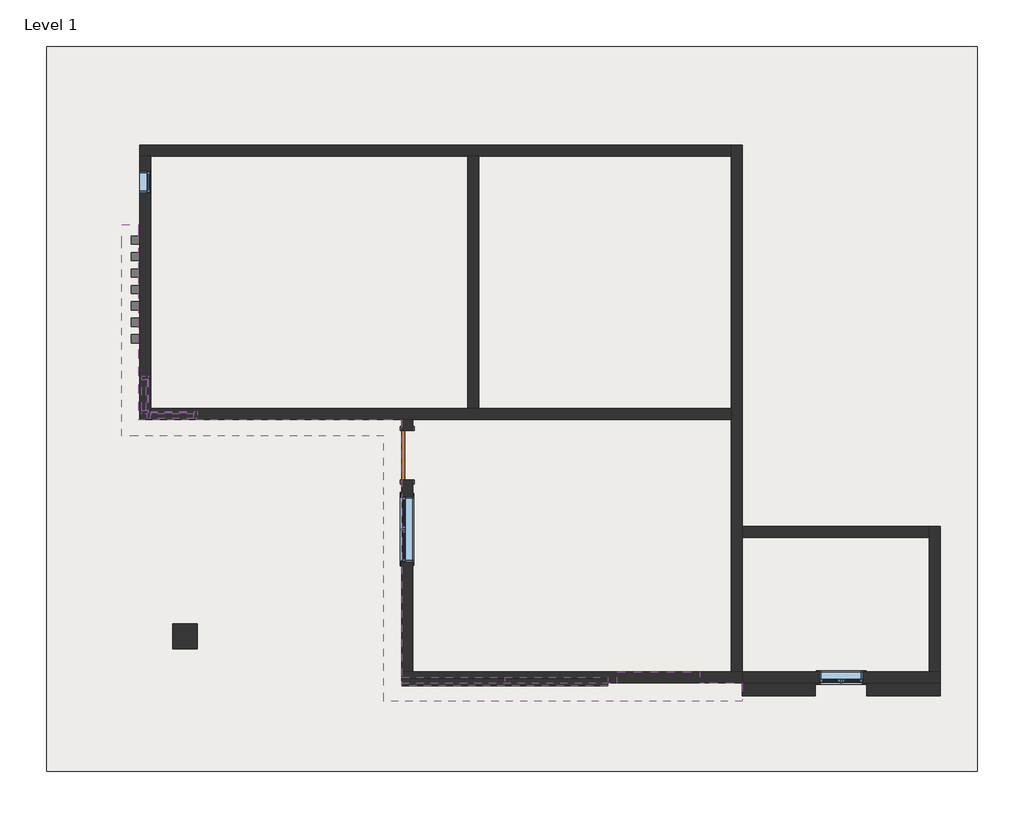
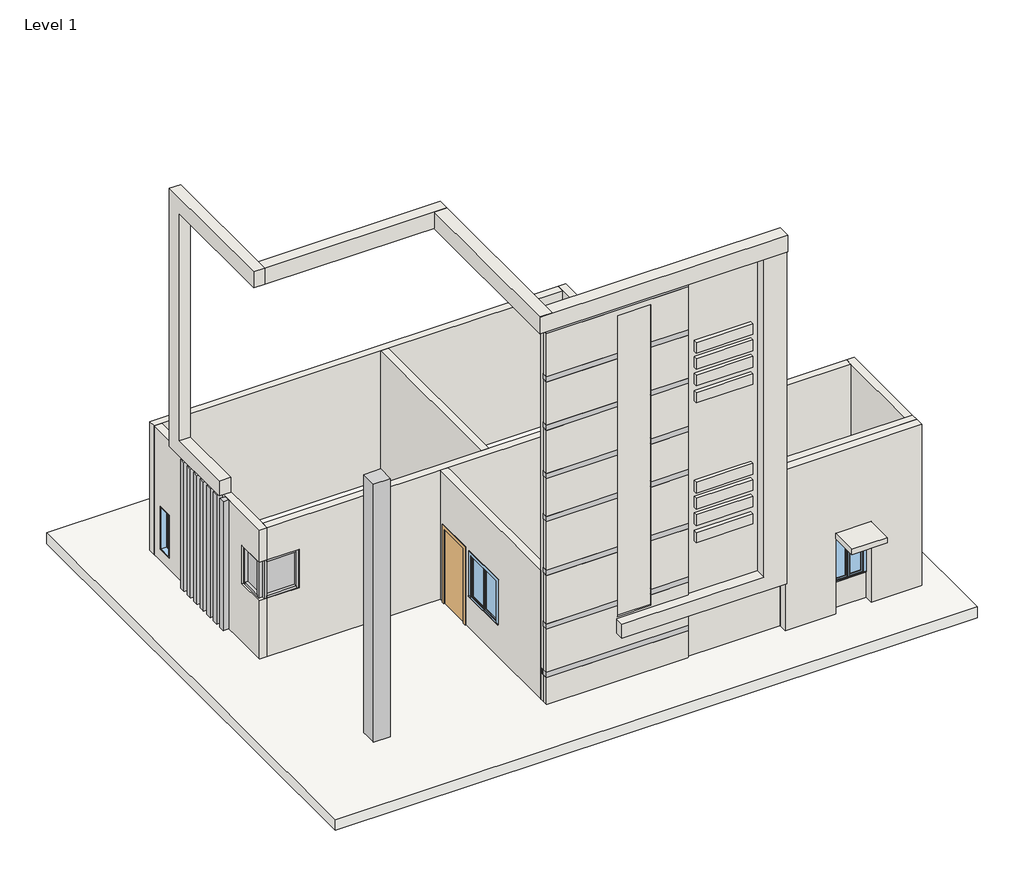
# One storey: 15 proxies, 13 walls, 8 members, 3 windows, 2 plates, 1 column, 1 door, 1 slab.
"""IFC4 building model written with IfcOpenShell, lengths in millimetres."""

from ifc_helpers import new_model, si_unit, frame, origin, origin_with_axes, place, context, project, spatial, polyline, outline, extrude, faceted_brep, transform, mapped, element, save
from components import column_b90849dc, door_54dd4da4, member_b7f4e0be, member_830eb86c, member_273a15f2, system_panel_glazed_3918bd16, system_panel_glazed_52a3cc88, walls_2_walls_2_327077e9, walls_3_walls_3_bd47f883, window_bb17773d, window_0862ab64, window_f81341e8

model = new_model("IFC4")

# Units and contexts
model_context = context("Model", 3, world=origin())
ifc_project = project(units=[si_unit("LENGTHUNIT", "METRE", prefix="MILLI")], contexts=[model_context])

# Site, building, storey
site = spatial("IfcSite", under=ifc_project)
building = spatial("IfcBuilding", under=site)
storey = spatial("IfcBuildingStorey", under=building, Name="Level 1", Elevation=0.0)

# Proxies
placement = place(None, origin())
element("IfcBuildingElementProxy", 1, Name="Cornice", ObjectType="Cornice", at=placement, inside=storey, context=model_context, shape_type="SweptSolid", body=[
    extrude(outline(polyline([(-12531.0681702, 7469.1112165), (-12683.4681702, 7469.1112165), (-12683.4681702, 7621.5112165), (-12531.0681702, 7621.5112165), (-12531.0681702, 7469.1112165)])), origin_with_axes(), (0.0, 0.0, 1.0), 3657.6),
])
element("IfcBuildingElementProxy", 2, Name="Cornice", ObjectType="Cornice", at=placement, inside=storey, context=model_context, shape_type="SweptSolid", body=[
    extrude(outline(polyline([(-12531.0681702, 7164.3112165), (-12683.4681702, 7164.3112165), (-12683.4681702, 7316.7112165), (-12531.0681702, 7316.7112165), (-12531.0681702, 7164.3112165)])), origin_with_axes(), (0.0, 0.0, 1.0), 3657.6),
])
element("IfcBuildingElementProxy", 3, Name="Cornice", ObjectType="Cornice", at=placement, inside=storey, context=model_context, shape_type="SweptSolid", body=[
    extrude(outline(polyline([(-12531.0681702, 6859.5112165), (-12683.4681702, 6859.5112165), (-12683.4681702, 7011.9112165), (-12531.0681702, 7011.9112165), (-12531.0681702, 6859.5112165)])), origin_with_axes(), (0.0, 0.0, 1.0), 3657.6),
])
element("IfcBuildingElementProxy", 4, Name="Cornice", ObjectType="Cornice", at=placement, inside=storey, context=model_context, shape_type="SweptSolid", body=[
    extrude(outline(polyline([(-12531.0681702, 6554.7112165), (-12683.4681702, 6554.7112165), (-12683.4681702, 6707.1112165), (-12531.0681702, 6707.1112165), (-12531.0681702, 6554.7112165)])), origin_with_axes(), (0.0, 0.0, 1.0), 3657.6),
])
element("IfcBuildingElementProxy", 5, Name="Cornice", ObjectType="Cornice", at=placement, inside=storey, context=model_context, shape_type="SweptSolid", body=[
    extrude(outline(polyline([(-12531.0681702, 6249.9112165), (-12683.4681702, 6249.9112165), (-12683.4681702, 6402.3112165), (-12531.0681702, 6402.3112165), (-12531.0681702, 6249.9112165)])), origin_with_axes(), (0.0, 0.0, 1.0), 3657.6),
])
element("IfcBuildingElementProxy", 6, Name="Cornice", ObjectType="Cornice", at=placement, inside=storey, context=model_context, shape_type="SweptSolid", body=[
    extrude(outline(polyline([(-12531.0681702, 5945.1112165), (-12683.4681702, 5945.1112165), (-12683.4681702, 6097.5112165), (-12531.0681702, 6097.5112165), (-12531.0681702, 5945.1112165)])), origin_with_axes(), (0.0, 0.0, 1.0), 3657.6),
])
element("IfcBuildingElementProxy", 7, Name="Cornice", ObjectType="Cornice", at=placement, inside=storey, context=model_context, shape_type="SweptSolid", body=[
    extrude(outline(polyline([(-12531.0681702, 5640.3112165), (-12683.4681702, 5640.3112165), (-12683.4681702, 5792.7112165), (-12531.0681702, 5792.7112165), (-12531.0681702, 5640.3112165)])), origin_with_axes(), (0.0, 0.0, 1.0), 3657.6),
])
element("IfcBuildingElementProxy", 8, Name="Reveal", ObjectType="Reveal", at=placement, inside=storey, context=model_context, shape_type="SweptSolid", body=[
    extrude(outline(polyline([(-7679.6681702, -703.3387835), (-7679.6681702, -550.9387835), (-3869.6681702, -550.9387835), (-3869.6681702, -703.3387835), (-7679.6681702, -703.3387835)])), frame((0.0, 0.0, 10515.6), z_axis=(0.0, 0.0, 1.0), x_axis=(1.0, 0.0, 0.0)), (0.0, 0.0, 1.0), 152.4),
])
element("IfcBuildingElementProxy", 9, Name="Reveal", ObjectType="Reveal", at=placement, inside=storey, context=model_context, shape_type="SweptSolid", body=[
    extrude(outline(polyline([(-4860.2681702, -703.3387835), (-4860.2681702, -550.9387835), (-3869.6681702, -550.9387835), (-3869.6681702, -703.3387835), (-4860.2681702, -703.3387835)])), frame((0.0, 0.0, 9144.0), z_axis=(0.0, 0.0, 1.0), x_axis=(1.0, 0.0, 0.0)), (0.0, 0.0, 1.0), 152.4),
    extrude(outline(polyline([(-7679.6681702, -703.3387835), (-7679.6681702, -550.9387835), (-5774.6681702, -550.9387835), (-5774.6681702, -703.3387835), (-7679.6681702, -703.3387835)])), frame((0.0, 0.0, 9144.0), z_axis=(0.0, 0.0, 1.0), x_axis=(1.0, 0.0, 0.0)), (0.0, 0.0, 1.0), 152.4),
])
element("IfcBuildingElementProxy", 10, Name="Reveal", ObjectType="Reveal", at=placement, inside=storey, context=model_context, shape_type="SweptSolid", body=[
    extrude(outline(polyline([(-4860.2681702, -703.3387835), (-4860.2681702, -550.9387835), (-3869.6681702, -550.9387835), (-3869.6681702, -703.3387835), (-4860.2681702, -703.3387835)])), frame((0.0, 0.0, 7772.4), z_axis=(0.0, 0.0, 1.0), x_axis=(1.0, 0.0, 0.0)), (0.0, 0.0, 1.0), 152.4),
    extrude(outline(polyline([(-7679.6681702, -703.3387835), (-7679.6681702, -550.9387835), (-5774.6681702, -550.9387835), (-5774.6681702, -703.3387835), (-7679.6681702, -703.3387835)])), frame((0.0, 0.0, 7772.4), z_axis=(0.0, 0.0, 1.0), x_axis=(1.0, 0.0, 0.0)), (0.0, 0.0, 1.0), 152.4),
])
element("IfcBuildingElementProxy", 11, Name="Reveal", ObjectType="Reveal", at=placement, inside=storey, context=model_context, shape_type="SweptSolid", body=[
    extrude(outline(polyline([(-4860.2681702, -703.3387835), (-4860.2681702, -550.9387835), (-3869.6681702, -550.9387835), (-3869.6681702, -703.3387835), (-4860.2681702, -703.3387835)])), frame((0.0, 0.0, 6400.8), z_axis=(0.0, 0.0, 1.0), x_axis=(1.0, 0.0, 0.0)), (0.0, 0.0, 1.0), 152.4),
    extrude(outline(polyline([(-7679.6681702, -703.3387835), (-7679.6681702, -550.9387835), (-5774.6681702, -550.9387835), (-5774.6681702, -703.3387835), (-7679.6681702, -703.3387835)])), frame((0.0, 0.0, 6400.8), z_axis=(0.0, 0.0, 1.0), x_axis=(1.0, 0.0, 0.0)), (0.0, 0.0, 1.0), 152.4),
])
element("IfcBuildingElementProxy", 12, Name="Reveal", ObjectType="Reveal", at=placement, inside=storey, context=model_context, shape_type="SweptSolid", body=[
    extrude(outline(polyline([(-4860.2681702, -703.3387835), (-4860.2681702, -550.9387835), (-3869.6681702, -550.9387835), (-3869.6681702, -703.3387835), (-4860.2681702, -703.3387835)])), frame((0.0, 0.0, 5181.6), z_axis=(0.0, 0.0, 1.0), x_axis=(1.0, 0.0, 0.0)), (0.0, 0.0, 1.0), 152.4),
    extrude(outline(polyline([(-7679.6681702, -703.3387835), (-7679.6681702, -550.9387835), (-5774.6681702, -550.9387835), (-5774.6681702, -703.3387835), (-7679.6681702, -703.3387835)])), frame((0.0, 0.0, 5181.6), z_axis=(0.0, 0.0, 1.0), x_axis=(1.0, 0.0, 0.0)), (0.0, 0.0, 1.0), 152.4),
])
element("IfcBuildingElementProxy", 13, Name="Reveal", ObjectType="Reveal", at=placement, inside=storey, context=model_context, shape_type="SweptSolid", body=[
    extrude(outline(polyline([(-4860.2681702, -703.3387835), (-4860.2681702, -550.9387835), (-3869.6681702, -550.9387835), (-3869.6681702, -703.3387835), (-4860.2681702, -703.3387835)])), frame((0.0, 0.0, 3657.6), z_axis=(0.0, 0.0, 1.0), x_axis=(1.0, 0.0, 0.0)), (0.0, 0.0, 1.0), 152.4),
    extrude(outline(polyline([(-7679.6681702, -703.3387835), (-7679.6681702, -550.9387835), (-5774.6681702, -550.9387835), (-5774.6681702, -703.3387835), (-7679.6681702, -703.3387835)])), frame((0.0, 0.0, 3657.6), z_axis=(0.0, 0.0, 1.0), x_axis=(1.0, 0.0, 0.0)), (0.0, 0.0, 1.0), 152.4),
])
element("IfcBuildingElementProxy", 14, Name="Reveal", ObjectType="Reveal", at=placement, inside=storey, context=model_context, shape_type="SweptSolid", body=[
    extrude(outline(polyline([(-4860.2681702, -703.3387835), (-4860.2681702, -550.9387835), (-3869.6681702, -550.9387835), (-3869.6681702, -703.3387835), (-4860.2681702, -703.3387835)])), frame((0.0, 0.0, 2133.6), z_axis=(0.0, 0.0, 1.0), x_axis=(1.0, 0.0, 0.0)), (0.0, 0.0, 1.0), 152.4),
    extrude(outline(polyline([(-7679.6681702, -703.3387835), (-7679.6681702, -550.9387835), (-5774.6681702, -550.9387835), (-5774.6681702, -703.3387835), (-7679.6681702, -703.3387835)])), frame((0.0, 0.0, 2133.6), z_axis=(0.0, 0.0, 1.0), x_axis=(1.0, 0.0, 0.0)), (0.0, 0.0, 1.0), 152.4),
])
element("IfcBuildingElementProxy", 15, Name="Reveal", ObjectType="Reveal", at=placement, inside=storey, context=model_context, shape_type="SweptSolid", body=[
    extrude(outline(polyline([(-7679.6681702, -703.3387835), (-7679.6681702, -550.9387835), (-3869.6681702, -550.9387835), (-3869.6681702, -703.3387835), (-7679.6681702, -703.3387835)])), frame((0.0, 0.0, 762.0), z_axis=(0.0, 0.0, 1.0), x_axis=(1.0, 0.0, 0.0)), (0.0, 0.0, 1.0), 152.4),
    extrude(outline(polyline([(-7679.6681702, -652.5387835), (-7679.6681702, -500.1387835), (-3869.6681702, -500.1387835), (-3869.6681702, -652.5387835), (-7679.6681702, -652.5387835)])), frame((0.0, 0.0, 762.0), z_axis=(0.0, 0.0, 1.0), x_axis=(1.0, 0.0, 0.0)), (0.0, 0.0, 1.0), 152.4),
])

# Column
column_shape = column_b90849dc(model_context)
element("IfcColumn", 16, ObjectType="Rectangular Column : 18\" x 18\"", at=placement, inside=storey, context=model_context, shape_type="MappedRepresentation", body=[
    mapped(column_shape, transform((-11692.8681702, 211.0612165, 0.0), x_axis=(1.0, 0.0, 0.0), y_axis=(0.0, 1.0, 0.0), z_axis=(0.0, 0.0, 1.0))),
])

# Door
door_shape = door_54dd4da4(model_context)
element("IfcDoor", 17, ObjectType="Single-Flush : 36\" x 84\"", at=placement, inside=storey, context=model_context, shape_type="MappedRepresentation", body=[
    mapped(door_shape, transform((-7578.0681702, 3563.8612165, 0.0), x_axis=(0.0, 1.0, 0.0), y_axis=(-1.0, 0.0, 0.0), z_axis=(0.0, 0.0, 1.0))),
])

# Members
member_shape = member_b7f4e0be(model_context)
element("IfcMember", 18, ObjectType="Rectangular Mullion : 2.5\" x 5\" rectangular", at=placement, inside=storey, context=model_context, shape_type="MappedRepresentation", body=[
    mapped(member_shape, transform((-12327.8681702, 4306.8112165, 1651.0), x_axis=(0.0, 0.0, -1.0), y_axis=(0.0, -1.0, 0.0), z_axis=(-1.0, 0.0, 0.0))),
])
member_2_shape = member_830eb86c(model_context)
element("IfcMember", 19, ObjectType="Rectangular Mullion : 2.5\" x 5\" rectangular", at=placement, inside=storey, context=model_context, shape_type="MappedRepresentation", body=[
    mapped(member_2_shape, transform((-12429.4681702, 4967.2112165, 1651.0), x_axis=(0.0, 0.0, -1.0), y_axis=(-1.0, 0.0, 0.0), z_axis=(0.0, 1.0, 0.0))),
])
element("IfcMember", 20, ObjectType="Rectangular Mullion : 2.5\" x 5\" rectangular", at=placement, inside=storey, context=model_context, shape_type="MappedRepresentation", body=[
    mapped(member_2_shape, transform((-12429.4681702, 4389.3612165, 2743.2), x_axis=(0.0, 0.0, 1.0), y_axis=(-1.0, 0.0, 0.0), z_axis=(0.0, -1.0, 0.0))),
])
member_3_shape = member_273a15f2(model_context)
element("IfcMember", 21, ObjectType="Rectangular Mullion : 2.5\" x 5\" rectangular", at=placement, inside=storey, context=model_context, shape_type="MappedRepresentation", body=[
    mapped(member_3_shape, transform((-12391.3681702, 4306.8112165, 2743.2), x_axis=(-1.0, 0.0, 0.0), y_axis=(0.0, -1.0, 0.0), z_axis=(0.0, 0.0, 1.0))),
])
element("IfcMember", 22, ObjectType="Rectangular Mullion : 2.5\" x 5\" rectangular", at=placement, inside=storey, context=model_context, shape_type="MappedRepresentation", body=[
    mapped(member_3_shape, transform((-12429.4681702, 5030.7112165, 2743.2), x_axis=(0.0, 1.0, 0.0), y_axis=(-1.0, 0.0, 0.0), z_axis=(0.0, 0.0, 1.0))),
])
element("IfcMember", 23, ObjectType="Rectangular Mullion : 2.5\" x 5\" rectangular", at=placement, inside=storey, context=model_context, shape_type="MappedRepresentation", body=[
    mapped(member_3_shape, transform((-11465.1280612, 4306.8112165, 1651.0), x_axis=(1.0, 0.0, 0.0), y_axis=(0.0, -1.0, 0.0), z_axis=(0.0, 0.0, -1.0))),
])
element("IfcMember", 24, ObjectType="Rectangular Mullion : 2.5\" x 5\" rectangular", at=placement, inside=storey, context=model_context, shape_type="MappedRepresentation", body=[
    mapped(member_3_shape, transform((-12429.4681702, 4325.8612165, 1651.0), x_axis=(0.0, -1.0, 0.0), y_axis=(-1.0, 0.0, 0.0), z_axis=(0.0, 0.0, -1.0))),
])
element("IfcMember", 25, ObjectType="Rectangular Mullion : 2.5\" x 5\" rectangular", at=placement, inside=storey, context=model_context, shape_type="MappedRepresentation", body=[
    mapped(member_shape, transform((-11528.6280612, 4306.8112165, 2743.2), x_axis=(0.0, 0.0, 1.0), y_axis=(0.0, -1.0, 0.0), z_axis=(1.0, 0.0, 0.0))),
])

# Plates
system_panel_glazed_shape = system_panel_glazed_3918bd16(model_context)
element("IfcPlate", 26, ObjectType="System Panel : Glazed", at=placement, inside=storey, context=model_context, shape_type="MappedRepresentation", body=[
    mapped(system_panel_glazed_shape, transform((-12429.4681702, 4678.2862165, 1714.5), x_axis=(0.0, -1.0, 0.0), y_axis=(1.0, 0.0, 0.0), z_axis=(0.0, 0.0, 1.0))),
])
system_panel_glazed_2_shape = system_panel_glazed_52a3cc88(model_context)
element("IfcPlate", 27, ObjectType="System Panel : Glazed", at=placement, inside=storey, context=model_context, shape_type="MappedRepresentation", body=[
    mapped(system_panel_glazed_2_shape, transform((-11928.2481157, 4306.8112165, 1714.5), x_axis=(1.0, 0.0, 0.0), y_axis=(0.0, 1.0, 0.0), z_axis=(0.0, 0.0, 1.0))),
])

# Slab
element("IfcSlab", 28, ObjectType="Generic - 12\"", at=placement, inside=storey, context=model_context, shape_type="SweptSolid", body=[
    extrude(outline(polyline([(2969.2570646, 11128.098465), (2969.2570646, -2283.101535), (-14251.9429354, -2283.101535), (-14251.9429354, 11128.098465), (2969.2570646, 11128.098465)])), frame((0.0, 0.0, -304.8), z_axis=(0.0, 0.0, 1.0), x_axis=(1.0, 0.0, 0.0)), (0.0, 0.0, 1.0), 304.8),
])

# Walls
element("IfcWall", 29, ObjectType="Generic - 5\"", at=placement, inside=storey, context=model_context, shape_type="SweptSolid", body=[
    extrude(outline(polyline([(-3869.6681702, -703.3387835), (-7679.6681702, -703.3387835), (-7679.6681702, -576.3387835), (-3869.6681702, -576.3387835), (-3869.6681702, -703.3387835)])), origin_with_axes(), (0.0, 0.0, 1.0), 762.0),
    extrude(outline(polyline([(-3869.6681702, -703.3387835), (-7679.6681702, -703.3387835), (-7679.6681702, -576.3387835), (-3869.6681702, -576.3387835), (-3869.6681702, -703.3387835)])), frame((0.0, 0.0, 10668.0), z_axis=(0.0, 0.0, 1.0), x_axis=(1.0, 0.0, 0.0)), (0.0, 0.0, 1.0), 304.8),
    extrude(outline(polyline([(1828.8, -4860.2681702), (1828.8, -5774.6681702), (2133.6, -5774.6681702), (2133.6, -7679.6681702), (914.4, -7679.6681702), (914.4, -3869.6681702), (2133.6, -3869.6681702), (2133.6, -4860.2681702), (1828.8, -4860.2681702)])), frame((0.0, -703.3387835, 0.0), z_axis=(0.0, 1.0, 0.0), x_axis=(0.0, 0.0, 1.0)), (0.0, 0.0, 1.0), 127.0),
    extrude(outline(polyline([(10363.2, -5774.6681702), (10363.2, -4860.2681702), (9296.4, -4860.2681702), (9296.4, -3869.6681702), (10515.6, -3869.6681702), (10515.6, -7679.6681702), (9296.4, -7679.6681702), (9296.4, -5774.6681702), (10363.2, -5774.6681702)])), frame((0.0, -703.3387835, 0.0), z_axis=(0.0, 1.0, 0.0), x_axis=(0.0, 0.0, 1.0)), (0.0, 0.0, 1.0), 127.0),
    extrude(outline(polyline([(-3869.6681702, -703.3387835), (-4860.2681702, -703.3387835), (-4860.2681702, -576.3387835), (-3869.6681702, -576.3387835), (-3869.6681702, -703.3387835)])), frame((0.0, 0.0, 7924.8), z_axis=(0.0, 0.0, 1.0), x_axis=(1.0, 0.0, 0.0)), (0.0, 0.0, 1.0), 1219.2),
    extrude(outline(polyline([(-5774.6681702, -703.3387835), (-7679.6681702, -703.3387835), (-7679.6681702, -576.3387835), (-5774.6681702, -576.3387835), (-5774.6681702, -703.3387835)])), frame((0.0, 0.0, 7924.8), z_axis=(0.0, 0.0, 1.0), x_axis=(1.0, 0.0, 0.0)), (0.0, 0.0, 1.0), 1219.2),
    extrude(outline(polyline([(-3869.6681702, -703.3387835), (-4860.2681702, -703.3387835), (-4860.2681702, -576.3387835), (-3869.6681702, -576.3387835), (-3869.6681702, -703.3387835)])), frame((0.0, 0.0, 6553.2), z_axis=(0.0, 0.0, 1.0), x_axis=(1.0, 0.0, 0.0)), (0.0, 0.0, 1.0), 1219.2),
    extrude(outline(polyline([(-5774.6681702, -703.3387835), (-7679.6681702, -703.3387835), (-7679.6681702, -576.3387835), (-5774.6681702, -576.3387835), (-5774.6681702, -703.3387835)])), frame((0.0, 0.0, 6553.2), z_axis=(0.0, 0.0, 1.0), x_axis=(1.0, 0.0, 0.0)), (0.0, 0.0, 1.0), 1219.2),
    extrude(outline(polyline([(-3869.6681702, -703.3387835), (-4860.2681702, -703.3387835), (-4860.2681702, -576.3387835), (-3869.6681702, -576.3387835), (-3869.6681702, -703.3387835)])), frame((0.0, 0.0, 5334.0), z_axis=(0.0, 0.0, 1.0), x_axis=(1.0, 0.0, 0.0)), (0.0, 0.0, 1.0), 1066.8),
    extrude(outline(polyline([(-5774.6681702, -703.3387835), (-7679.6681702, -703.3387835), (-7679.6681702, -576.3387835), (-5774.6681702, -576.3387835), (-5774.6681702, -703.3387835)])), frame((0.0, 0.0, 5334.0), z_axis=(0.0, 0.0, 1.0), x_axis=(1.0, 0.0, 0.0)), (0.0, 0.0, 1.0), 1066.8),
    extrude(outline(polyline([(-3869.6681702, -703.3387835), (-4860.2681702, -703.3387835), (-4860.2681702, -576.3387835), (-3869.6681702, -576.3387835), (-3869.6681702, -703.3387835)])), frame((0.0, 0.0, 3810.0), z_axis=(0.0, 0.0, 1.0), x_axis=(1.0, 0.0, 0.0)), (0.0, 0.0, 1.0), 1371.6),
    extrude(outline(polyline([(-5774.6681702, -703.3387835), (-7679.6681702, -703.3387835), (-7679.6681702, -576.3387835), (-5774.6681702, -576.3387835), (-5774.6681702, -703.3387835)])), frame((0.0, 0.0, 3810.0), z_axis=(0.0, 0.0, 1.0), x_axis=(1.0, 0.0, 0.0)), (0.0, 0.0, 1.0), 1371.6),
    extrude(outline(polyline([(-3869.6681702, -703.3387835), (-4860.2681702, -703.3387835), (-4860.2681702, -576.3387835), (-3869.6681702, -576.3387835), (-3869.6681702, -703.3387835)])), frame((0.0, 0.0, 2286.0), z_axis=(0.0, 0.0, 1.0), x_axis=(1.0, 0.0, 0.0)), (0.0, 0.0, 1.0), 1371.6),
    extrude(outline(polyline([(-5774.6681702, -703.3387835), (-7679.6681702, -703.3387835), (-7679.6681702, -576.3387835), (-5774.6681702, -576.3387835), (-5774.6681702, -703.3387835)])), frame((0.0, 0.0, 2286.0), z_axis=(0.0, 0.0, 1.0), x_axis=(1.0, 0.0, 0.0)), (0.0, 0.0, 1.0), 1371.6),
])
element("IfcWall", 30, ObjectType="Generic - 8\"", at=placement, inside=storey, context=model_context, shape_type="Brep", body=[
    faceted_brep([(-12531.0681702, 9101.0612165, 0.0), (-12327.8681702, 9101.0612165, 0.0), (-6460.4681702, 9101.0612165, 0.0), (-6257.2681702, 9101.0612165, 0.0), (-1583.6681702, 9101.0612165, 0.0), (-1583.6681702, 9101.0612165, 3657.6), (-6257.2681702, 9101.0612165, 3657.6), (-6460.4681702, 9101.0612165, 3657.6), (-12327.8681702, 9101.0612165, 3657.6), (-12531.0681702, 9101.0612165, 3657.6), (-12531.0681702, 9304.2612165, 0.0), (-12531.0681702, 9304.2612165, 3657.6), (-1583.6681702, 9304.2612165, 3657.6), (-1583.6681702, 9304.2612165, 0.0)], [[[0, 1, 2, 3, 4, 5, 6, 7, 8, 9]], [[10, 11, 12, 13]], [[4, 3, 2, 1, 0, 10, 13]], [[0, 9, 11, 10]], [[5, 4, 13, 12]], [[9, 8, 7, 6, 5, 12, 11]]]),
])
element("IfcWall", 31, ObjectType="Generic - 8\"", at=placement, inside=storey, context=model_context, shape_type="Brep", body=[
    faceted_brep([(-12327.8681702, 9101.0612165, 0.0), (-12327.8681702, 9101.0612165, 3657.6), (-12327.8681702, 4427.4612165, 3657.6), (-12327.8681702, 4224.2612165, 3657.6), (-12327.8681702, 4224.2612165, 2743.2), (-12327.8681702, 4427.4612165, 2743.2), (-12327.8681702, 5030.7112165, 2743.2), (-12327.8681702, 5030.7112165, 1651.0), (-12327.8681702, 4427.4612165, 1651.0), (-12327.8681702, 4224.2612165, 1651.0), (-12327.8681702, 4224.2612165, 0.0), (-12327.8681702, 4427.4612165, 0.0), (-12327.8681702, 8415.2612165, 1544.9460414), (-12327.8681702, 8821.6612165, 1544.9460414), (-12327.8681702, 8821.6612165, 325.7460414), (-12327.8681702, 8415.2612165, 325.7460414), (-12531.0681702, 9101.0612165, 0.0), (-12531.0681702, 4224.2612165, 0.0), (-12531.0681702, 4224.2612165, 1651.0), (-12531.0681702, 5030.7112165, 1651.0), (-12531.0681702, 5030.7112165, 2743.2), (-12531.0681702, 4224.2612165, 2743.2), (-12531.0681702, 4224.2612165, 3657.6), (-12531.0681702, 9101.0612165, 3657.6), (-12531.0681702, 8415.2612165, 1544.9460414), (-12531.0681702, 8415.2612165, 325.7460414), (-12531.0681702, 8821.6612165, 325.7460414), (-12531.0681702, 8821.6612165, 1544.9460414)], [[[0, 1, 2, 3, 4, 5, 6, 7, 8, 9, 10, 11], [12, 13, 14, 15]], [[16, 17, 18, 19, 20, 21, 22, 23], [24, 25, 26, 27]], [[1, 0, 16, 23]], [[3, 2, 1, 23, 22]], [[0, 11, 10, 17, 16]], [[6, 5, 4, 21, 20]], [[7, 6, 20, 19]], [[9, 8, 7, 19, 18]], [[10, 9, 18, 17]], [[4, 3, 22, 21]], [[25, 24, 12, 15]], [[26, 25, 15, 14]], [[27, 26, 14, 13]], [[24, 27, 13, 12]]]),
])
element("IfcWall", 32, ObjectType="Generic - 8\"", at=placement, inside=storey, context=model_context, shape_type="Brep", body=[
    faceted_brep([(-1583.6681702, 9304.2612165, 0.0), (-1583.6681702, 9101.0612165, 0.0), (-1583.6681702, 4427.4612165, 0.0), (-1583.6681702, 4224.2612165, 0.0), (-1583.6681702, -449.3387835, 0.0), (-1583.6681702, -449.3387835, 3657.6), (-1583.6681702, 4224.2612165, 3657.6), (-1583.6681702, 4427.4612165, 3657.6), (-1583.6681702, 9101.0612165, 3657.6), (-1583.6681702, 9304.2612165, 3657.6), (-1380.4681702, 9304.2612165, 0.0), (-1380.4681702, 9304.2612165, 3657.6), (-1380.4681702, -449.3387835, 3657.6), (-1380.4681702, -449.3387835, 0.0), (-1380.4681702, 2039.8612165, 0.0), (-1380.4681702, 2243.0612165, 0.0)], [[[0, 1, 2, 3, 4, 5, 6, 7, 8, 9]], [[10, 11, 12, 13, 14, 15]], [[4, 3, 2, 1, 0, 10, 15, 14, 13]], [[0, 9, 11, 10]], [[9, 8, 7, 6, 5, 12, 11]], [[5, 4, 13, 12]]]),
])
element("IfcWall", 33, ObjectType="Generic - 8\"", at=placement, inside=storey, context=model_context, shape_type="Brep", body=[
    faceted_brep([(-7679.6681702, 4224.2612165, 0.0), (-7679.6681702, 4021.0612165, 0.0), (-7679.6681702, 4021.0612165, 2133.6), (-7679.6681702, 3106.6612165, 2133.6), (-7679.6681702, 3106.6612165, 0.0), (-7679.6681702, -449.3387835, 0.0), (-7679.6681702, -449.3387835, 3657.6), (-7679.6681702, 3182.8612165, 3657.6), (-7679.6681702, 4097.2612165, 3657.6), (-7679.6681702, 4224.2612165, 3657.6), (-7679.6681702, 2801.8612165, 2133.6), (-7679.6681702, 1582.6612165, 2133.6), (-7679.6681702, 1582.6612165, 914.4), (-7679.6681702, 2801.8612165, 914.4), (-7476.4681702, 4021.0612165, 2133.6), (-7476.4681702, 4021.0612165, 0.0), (-7476.4681702, 4224.2612165, 0.0), (-7476.4681702, 4224.2612165, 3657.6), (-7476.4681702, 4097.2612165, 3657.6), (-7476.4681702, 3182.8612165, 3657.6), (-7476.4681702, -449.3387835, 3657.6), (-7476.4681702, -449.3387835, 0.0), (-7476.4681702, 3106.6612165, 0.0), (-7476.4681702, 3106.6612165, 2133.6), (-7476.4681702, 2801.8612165, 2133.6), (-7476.4681702, 2801.8612165, 914.4), (-7476.4681702, 1582.6612165, 914.4), (-7476.4681702, 1582.6612165, 2133.6)], [[[0, 1, 2, 3, 4, 5, 6, 7, 8, 9], [10, 11, 12, 13]], [[14, 15, 16, 17, 18, 19, 20, 21, 22, 23], [24, 25, 26, 27]], [[22, 21, 5, 4]], [[16, 15, 1, 0]], [[0, 9, 17, 16]], [[9, 8, 7, 6, 20, 19, 18, 17]], [[6, 5, 21, 20]], [[25, 24, 10, 13]], [[26, 25, 13, 12]], [[27, 26, 12, 11]], [[24, 27, 11, 10]], [[2, 1, 15, 14]], [[3, 2, 14, 23]], [[4, 3, 23, 22]]]),
])
element("IfcWall", 34, ObjectType="Generic - 8\"", at=placement, inside=storey, context=model_context, shape_type="Brep", body=[
    faceted_brep([(-1583.6681702, 4224.2612165, 0.0), (-1583.6681702, 4224.2612165, 3657.6), (-7476.4681702, 4224.2612165, 3657.6), (-7679.6681702, 4224.2612165, 3657.6), (-12327.8681702, 4224.2612165, 3657.6), (-12327.8681702, 4224.2612165, 2743.2), (-11465.1280612, 4224.2612165, 2743.2), (-11465.1280612, 4224.2612165, 1651.0), (-12327.8681702, 4224.2612165, 1651.0), (-12327.8681702, 4224.2612165, 0.0), (-7679.6681702, 4224.2612165, 0.0), (-7476.4681702, 4224.2612165, 0.0), (-1583.6681702, 4427.4612165, 0.0), (-6257.2681702, 4427.4612165, 0.0), (-6460.4681702, 4427.4612165, 0.0), (-12327.8681702, 4427.4612165, 0.0), (-12327.8681702, 4427.4612165, 1651.0), (-11465.1280612, 4427.4612165, 1651.0), (-11465.1280612, 4427.4612165, 2743.2), (-12327.8681702, 4427.4612165, 2743.2), (-12327.8681702, 4427.4612165, 3657.6), (-6460.4681702, 4427.4612165, 3657.6), (-6257.2681702, 4427.4612165, 3657.6), (-1583.6681702, 4427.4612165, 3657.6)], [[[0, 1, 2, 3, 4, 5, 6, 7, 8, 9, 10, 11]], [[12, 13, 14, 15, 16, 17, 18, 19, 20, 21, 22, 23]], [[1, 0, 12, 23]], [[4, 3, 2, 1, 23, 22, 21, 20]], [[0, 11, 10, 9, 15, 14, 13, 12]], [[6, 5, 19, 18]], [[7, 6, 18, 17]], [[8, 7, 17, 16]], [[9, 8, 16, 15]], [[5, 4, 20, 19]]]),
])
element("IfcWall", 35, ObjectType="Generic - 8\"", at=placement, inside=storey, context=model_context, shape_type="SweptSolid", body=[
    extrude(outline(polyline([(-6460.4681702, 4427.4612165), (-6460.4681702, 9101.0612165), (-6257.2681702, 9101.0612165), (-6257.2681702, 4427.4612165), (-6460.4681702, 4427.4612165)])), origin_with_axes(), (0.0, 0.0, 1.0), 3657.6),
])
element("IfcWall", 36, ObjectType="Generic - 8\"", at=placement, inside=storey, context=model_context, shape_type="Brep", body=[
    faceted_brep([(-7679.6681702, -652.5387835, 0.0), (-1380.4681702, -652.5387835, 0.0), (-1380.4681702, -652.5387835, 4572.0), (-1380.4681702, -652.5387835, 10972.8), (-7679.6681702, -652.5387835, 10972.8), (-7679.6681702, -652.5387835, 914.4), (-3869.6681702, -652.5387835, 914.4), (-3869.6681702, -652.5387835, 762.0), (-7679.6681702, -652.5387835, 762.0), (-1380.4681702, -449.3387835, 0.0), (-1583.6681702, -449.3387835, 0.0), (-7476.4681702, -449.3387835, 0.0), (-7679.6681702, -449.3387835, 0.0), (-7679.6681702, -449.3387835, 3657.6), (-7679.6681702, -449.3387835, 7315.2), (-7679.6681702, -449.3387835, 10972.8), (-7476.4681702, -449.3387835, 10972.8), (-1583.6681702, -449.3387835, 10972.8), (-1380.4681702, -449.3387835, 10972.8), (-1380.4681702, -449.3387835, 7315.2), (-1380.4681702, -449.3387835, 4572.0), (-1380.4681702, -449.3387835, 3657.6), (-7679.6681702, -500.1387835, 762.0), (-7679.6681702, -500.1387835, 914.4), (-3869.6681702, -500.1387835, 762.0), (-3869.6681702, -500.1387835, 914.4)], [[[0, 1, 2, 3, 4, 5, 6, 7, 8]], [[9, 10, 11, 12, 13, 14, 15, 16, 17, 18, 19, 20, 21]], [[1, 0, 12, 11, 10, 9]], [[12, 0, 8, 22, 23, 5, 4, 15, 14, 13]], [[4, 3, 18, 17, 16, 15]], [[24, 7, 6, 25]], [[25, 6, 5, 23]], [[24, 25, 23, 22]], [[7, 24, 22, 8]], [[1, 9, 21, 20, 19, 18, 3, 2]]]),
])
element("IfcWall", 37, ObjectType="Generic - 8\"", at=placement, inside=storey, context=model_context, shape_type="Brep", body=[
    faceted_brep([(-1380.4681702, -652.5387835, 4572.0), (-1380.4681702, -652.5387835, 0.0), (2277.1318298, -652.5387835, 0.0), (2277.1318298, -652.5387835, 4572.0), (41.9318298, -652.5387835, 1955.8), (854.7318298, -652.5387835, 1955.8), (854.7318298, -652.5387835, 736.6), (41.9318298, -652.5387835, 736.6), (-1380.4681702, -449.3387835, 0.0), (-1380.4681702, -449.3387835, 4572.0), (2073.9318298, -449.3387835, 4572.0), (2277.1318298, -449.3387835, 4572.0), (2277.1318298, -449.3387835, 0.0), (2073.9318298, -449.3387835, 0.0), (41.9318298, -449.3387835, 1955.8), (41.9318298, -449.3387835, 736.6), (854.7318298, -449.3387835, 736.6), (854.7318298, -449.3387835, 1955.8)], [[[0, 1, 2, 3], [4, 5, 6, 7]], [[8, 9, 10, 11, 12, 13], [14, 15, 16, 17]], [[2, 1, 8, 13, 12]], [[0, 3, 11, 10, 9]], [[0, 9, 8, 1]], [[3, 2, 12, 11]], [[15, 14, 4, 7]], [[16, 15, 7, 6]], [[17, 16, 6, 5]], [[14, 17, 5, 4]]]),
])
element("IfcWall", 38, ObjectType="Generic - 8\"", at=placement, inside=storey, context=model_context, shape_type="Brep", body=[
    faceted_brep([(2277.1318298, -449.3387835, 0.0), (2277.1318298, 2243.0612165, 0.0), (2277.1318298, 2243.0612165, 4572.0), (2277.1318298, -449.3387835, 4572.0), (2073.9318298, -449.3387835, 0.0), (2073.9318298, -449.3387835, 4572.0), (2073.9318298, 2039.8612165, 4572.0), (2073.9318298, 2243.0612165, 4572.0), (2073.9318298, 2243.0612165, 0.0), (2073.9318298, 2039.8612165, 0.0)], [[[0, 1, 2, 3]], [[4, 5, 6, 7, 8, 9]], [[1, 0, 4, 9, 8]], [[3, 2, 7, 6, 5]], [[0, 3, 5, 4]], [[2, 1, 8, 7]]]),
])
element("IfcWall", 39, ObjectType="Generic - 8\"", at=placement, inside=storey, context=model_context, shape_type="SweptSolid", body=[
    extrude(outline(polyline([(-1380.4681702, 2243.0612165), (2073.9318298, 2243.0612165), (2073.9318298, 2039.8612165), (-1380.4681702, 2039.8612165), (-1380.4681702, 2243.0612165)])), origin_with_axes(), (0.0, 0.0, 1.0), 4572.0),
])
walls_2_walls_2_shape = walls_2_walls_2_327077e9(model_context)
element("IfcWall", 40, ObjectType="Walls 2 : Walls 2", at=placement, inside=storey, context=model_context, shape_type="MappedRepresentation", body=[
    mapped(walls_2_walls_2_shape, transform((0.0, 0.0, 0.0), x_axis=(1.0, 0.0, 0.0), y_axis=(0.0, 1.0, 0.0), z_axis=(0.0, 0.0, 1.0))),
])
walls_3_walls_3_shape = walls_3_walls_3_bd47f883(model_context)
element("IfcWall", 41, ObjectType="Walls 3 : Walls 3", at=placement, inside=storey, context=model_context, shape_type="MappedRepresentation", body=[
    mapped(walls_3_walls_3_shape, transform((0.0, 0.0, 0.0), x_axis=(1.0, 0.0, 0.0), y_axis=(0.0, 1.0, 0.0), z_axis=(0.0, 0.0, 1.0))),
])

# Windows
window_shape = window_bb17773d(model_context)
element("IfcWindow", 42, ObjectType="Casement Dbl with Trim : 32\" x 48\"", at=placement, inside=storey, context=model_context, shape_type="MappedRepresentation", body=[
    mapped(window_shape, transform((448.3318298, -531.8887835, -177.8), x_axis=(-1.0, 0.0, 0.0), y_axis=(0.0, -1.0, 0.0), z_axis=(0.0, 0.0, 1.0))),
])
window_2_shape = window_0862ab64(model_context)
element("IfcWindow", 43, ObjectType="Casement Dbl with Trim : 48\" x 48\"", at=placement, inside=storey, context=model_context, shape_type="MappedRepresentation", body=[
    mapped(window_2_shape, transform((-7559.0181702, 2192.2612165, 0.0), x_axis=(0.0, 1.0, 0.0), y_axis=(-1.0, 0.0, 0.0), z_axis=(0.0, 0.0, 1.0))),
])
window_3_shape = window_f81341e8(model_context)
element("IfcWindow", 44, ObjectType="Fixed : 16\" x 48\"", at=placement, inside=storey, context=model_context, shape_type="MappedRepresentation", body=[
    mapped(window_3_shape, transform((-12429.4681702, 8580.3612165, -588.6539586), x_axis=(0.0, -1.0, 0.0), y_axis=(1.0, 0.0, 0.0), z_axis=(0.0, 0.0, 1.0))),
])

save(model, "model.ifc")

# Revit data of these elements
# Type "Rectangular Column : 18\" x 18\""
#   Assembly Code = "B1010200"
#   Depth = 1' - 6"
#   Offset Base = 0' - 0"
#   Offset Top = 0' - 0"
#   Width = 1' - 6"
#   Material = none
# Type "Single-Flush : 36\" x 84\""
#   Type Mark = "1"
#   Construction Type Id = "MDOOR"
#   Assembly Code = "C1020"
#   Analytic Construction = "Metal"
#   Thickness = 0' - 2"
#   Heat Transfer Coefficient (U) = 0.651978 BTU/(h·ft²·°F)
#   Height = 7' - 0"
#   Trim Projection Ext = 0' - 1"
#   Trim Projection Int = 0' - 1"
#   Trim Width = 0' - 3"
#   Width = 3' - 0"
#   Define Thermal Properties by = 1
#   Door Material = Door - Panel
#   Frame Material = Door - Frame
#   Visual Light Transmittance = 0
#   Solar Heat Gain Coefficient = 0
#   Function = (empty or 0)
#   Wall Closure = (empty or 0)
# Type "Rectangular Mullion : 2.5\" x 5\" rectangular"
#   built-in parameter 1007304 = 0.416667 (stored number, unit not read)
#   built-in parameter 1007301 = 0.104167 (stored number, unit not read)
#   built-in parameter 1007300 = 0.104167 (stored number, unit not read)
# Type "System Panel : Glazed"
#   Construction Type Id = "GSP4R"
#   Analytic Construction = "1/8 in Pilkington single glazing"
#   Visual Light Transmittance = 0.9
#   Solar Heat Gain Coefficient = 0.86
#   Heat Transfer Coefficient (U) = 1.18115 BTU/(h·ft²·°F)
# Type "Generic - 12\""
#   Assembly Code = "B1010"
#   Function = 0
#   Layers, outside or top first: 1' - 0" no material (function 1)
# Type "Generic - 5\""
#   Assembly Code = "B2010"
#   Layers, outside or top first: 0' - 5" no material (function 1)
# Type "Generic - 8\""
#   Assembly Code = "B2010"
#   Layers, outside or top first: 0' - 8" no material (function 1)
# Type "Casement Dbl with Trim : 32\" x 48\""
#   Type Mark = "15"
#   Construction Type Id = "GSP4R"
#   Assembly Code = "B2020100"
#   Analytic Construction = "1/8 in Pilkington single glazing"
#   Visual Light Transmittance = 0.9
#   Solar Heat Gain Coefficient = 0.78
#   Heat Transfer Coefficient (U) = 0.6496 BTU/(h·ft²·°F)
#   Height = 4' - 0"
#   Default Sill Height = 3' - 0"
#   Trim Projection - Ext. = 0' - 0 1/2"
#   Trim Projection - Int. = 0' - 0 3/4"
#   Trim Width - Exterior = 0' - 3 1/2"
#   Trim Width - Interior = 0' - 3 1/2"
#   Width = 2' - 8"
#   Window Inset = 0' - 0 3/4"
#   Define Thermal Properties by = 1
#   Glass Pane Material = Glass
#   Sash Material = Sash
#   Trim Exterior Material = Trim
#   Trim Interior Material = Trim
#   Wall Closure = (empty or 0)
# Type "Casement Dbl with Trim : 48\" x 48\""
#   Type Mark = "13"
#   Construction Type Id = "GSP4R"
#   Assembly Code = "B2020100"
#   Analytic Construction = "1/8 in Pilkington single glazing"
#   Visual Light Transmittance = 0.9
#   Solar Heat Gain Coefficient = 0.78
#   Heat Transfer Coefficient (U) = 0.6496 BTU/(h·ft²·°F)
#   Height = 4' - 0"
#   Default Sill Height = 3' - 0"
#   Trim Projection - Ext. = 0' - 0 1/2"
#   Trim Projection - Int. = 0' - 0 3/4"
#   Trim Width - Exterior = 0' - 3 1/2"
#   Trim Width - Interior = 0' - 3 1/2"
#   Width = 4' - 0"
#   Window Inset = 0' - 0 3/4"
#   Define Thermal Properties by = 1
#   Glass Pane Material = Glass
#   Sash Material = Sash
#   Trim Exterior Material = Trim
#   Trim Interior Material = Trim
#   Wall Closure = (empty or 0)
# Type "Fixed : 16\" x 48\""
#   Type Mark = "5"
#   Construction Type Id = "GSP4R"
#   Assembly Code = "B2020100"
#   Analytic Construction = "1/8 in Pilkington single glazing"
#   Visual Light Transmittance = 0.9
#   Solar Heat Gain Coefficient = 0.78
#   Heat Transfer Coefficient (U) = 0.6496 BTU/(h·ft²·°F)
#   Height = 4' - 0"
#   Default Sill Height = 3' - 0"
#   Width = 1' - 4"
#   Window Inset = 0' - 0 3/4"
#   Define Thermal Properties by = 1
#   Glass Pane Material = Glass
#   Sash Material = Sash
#   Wall Closure = (empty or 0)
# Elements 1, 2, 3, 4, 5, 6, 7 (IfcBuildingElementProxy, "Cornice")
#   Phase Created = New Construction
#   Materials on its faces: "Default Wall"
# Element 16 (IfcColumn, "Rectangular Column : 18\" x 18\"")
#   Phase Created = New Construction
# Element 17 (IfcDoor, "Single-Flush : 36\" x 84\"")
#   Phase Created = New Construction
#   Materials on its faces: "Door - Frame", "Door - Panel"
# Elements 18, 19, 20, 21, 22, 23, 24, 25 (IfcMember, "Rectangular Mullion : 2.5\" x 5\" rectangular")
#   Phase Created = New Construction
#   Materials on its faces: "Aluminum"
# Elements 26, 27 (IfcPlate, "System Panel : Glazed")
#   Phase Created = New Construction
#   Materials on its faces: "Glass"
# Element 28 (IfcSlab, "Generic - 12\"")
#   Height Offset From Level = 0' - 0"
#   Phase Created = New Construction
#   Materials on its faces: "Default Floor"
# Element 29 (IfcWall, "Generic - 5\"")
#   Top Offset = 24' - 0"
#   Base Offset = 0' - 0"
#   wall height = 36' - 0"
#   Phase Created = New Construction
#   Base Constraint = Level 1
#   Top Constraint = Level 2
#   Materials on its faces: "Default Wall"
# Elements 30, 31, 32, 33, 34, 35 (IfcWall, "Generic - 8\"")
#   Top Offset = 0' - 0"
#   Base Offset = 0' - 0"
#   Unconnected Height = 12' - 0"
#   wall height = 12' - 0"
#   Phase Created = New Construction
#   Base Constraint = Level 1
#   Materials on its faces: "Default Wall"
# Element 36 (IfcWall, "Generic - 8\"")
#   Top Offset = 0' - 0"
#   Base Offset = 0' - 0"
#   Unconnected Height = 36' - 0"
#   wall height = 36' - 0"
#   Phase Created = New Construction
#   Base Constraint = Level 1
#   Materials on its faces: "Default Wall"
# Elements 37, 38, 39 (IfcWall, "Generic - 8\"")
#   Top Offset = 0' - 0"
#   Base Offset = 0' - 0"
#   Unconnected Height = 15' - 0"
#   wall height = 15' - 0"
#   Phase Created = New Construction
#   Base Constraint = Level 1
#   Materials on its faces: "Default Wall"
# Element 40 (IfcWall, "Walls 2 : Walls 2")
#   Phase Created = New Construction
#   Materials on its faces: "Default Wall"
# Element 41 (IfcWall, "Walls 3 : Walls 3")
#   Phase Created = New Construction
#   Materials on its faces: "Default Wall"
# Element 42 (IfcWindow, "Casement Dbl with Trim : 32\" x 48\"")
#   Mark = "6"
#   Phase Created = New Construction
#   Materials on its faces: "Sash", "Trim", "Glass"
# Element 43 (IfcWindow, "Casement Dbl with Trim : 48\" x 48\"")
#   Mark = "3"
#   Phase Created = New Construction
#   Materials on its faces: "Sash", "Trim", "Glass"
# Element 44 (IfcWindow, "Fixed : 16\" x 48\"")
#   Mark = "7"
#   Phase Created = New Construction
#   Materials on its faces: "Sash", "Glass"
# Materials
#   "Door - Panel": class "Wood", colour RGB 210 159 95, transparency 0
#   "Door - Frame": colour RGB 118 70 51, transparency 0
#   "Glass": class "Glass", colour RGB 0 128 192, transparency 0.75, Description = "Soda Lime Glass", Cost = 0
#   "Sash": class "Wood", colour RGB 224 178 126, transparency 0
#   "Trim": class "Wood", colour RGB 224 178 126, transparency 0
#   "Default Wall": colour RGB 128 128 128, transparency 0
#   "Aluminum": class "Metal", colour RGB 247 247 247, transparency 0, Description = "Aluminum 6061", Cost = 0
#   "Default Floor": colour RGB 128 128 128, transparency 0
